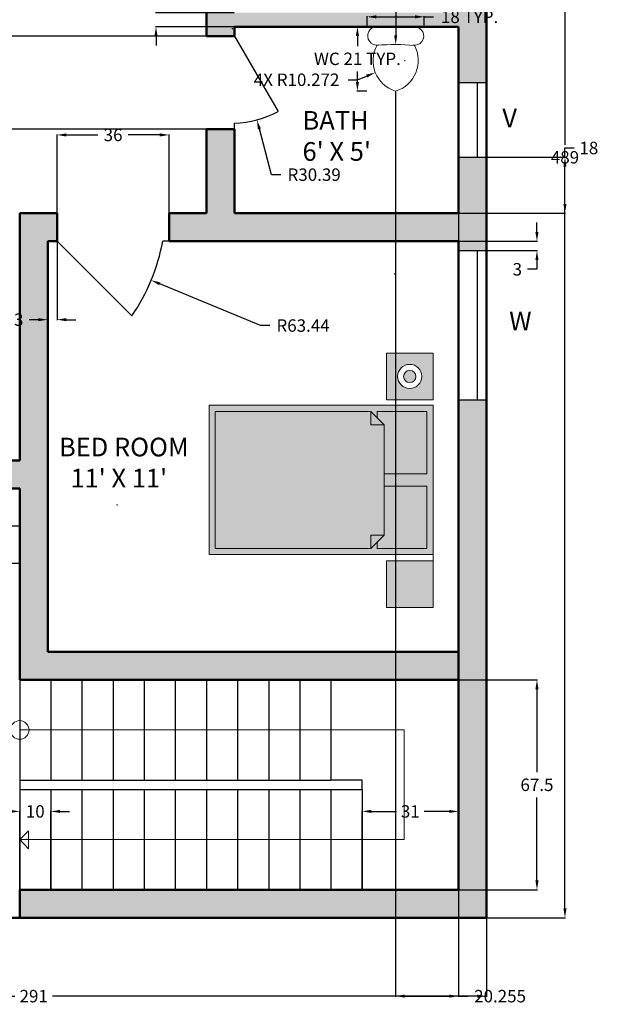
# Model space of a CAD drawing. Units: inches. Extents: x 30 to 385, y 81 to 626.
# Tile 2 of 4: x 199 to 385, y 81 to 398. Entities that reach past the tile are written whole.
import ezdxf

# ---------------------------------------------------------------- set-up
doc = ezdxf.new("R2010")
doc.units = ezdxf.units.IN
doc.header["$MEASUREMENT"] = 0
for name, color, linetype, lineweight in [('A-ANNO-DIMS', 2, 'Continuous', 18), ('A-ANNO-SYMB', 7, 'Continuous', 18), ('A-ANNO-TEXT', 7, 'Continuous', 18), ('A-AREA-IDEN', 7, 'Continuous', 25), ('A-DOOR', 3, 'Continuous', 25), ('A-FLOR-FIXT', 8, 'Continuous', 18), ('A-FLOR-STRS', 7, 'Continuous', 25), ('A-FURN', 8, 'Continuous', 18), ('A-GLAZ', 4, 'Continuous', 25), ('A-WALL', 7, 'Continuous', 50), ('A-WALL-PATT', 32, 'Continuous', 13)]:
    doc.layers.add(name, color=color, linetype=linetype, lineweight=lineweight)
doc.layers.add('A-FURN-PATT', color=254, linetype='Continuous', lineweight=13, true_color=0xfeeab9)
doc.styles.get("Standard").update_dxf_attribs({"font": 'arial.ttf'})
doc.dimstyles.get("Standard").update_dxf_attribs({"dimtxt": 4, "dimasz": 3, "dimexe": 0.18, "dimexo": 0.0625, "dimgap": 2, "dimtad": 0, "dimtih": 1, "dimtoh": 1, "dimdec": 0, "dimzin": 0, "dimdsep": 46, "dimlunit": 3, "dimtxsty": 'Standard', "dimcen": 0.09, "dimadec": 0, "dimazin": 0, "dimtfac": 1, "dimtdec": 0, "dimtofl": 0, "dimtmove": 0, "dimatfit": 3, "dimfxl": 1, "dimtolj": 1, "dimtzin": 0, "dimarcsym": 0})

# ---------------------------------------------------------------- blocks, each defined once
blk = doc.blocks.new('WIN-48')
for p, q in [((0, 0), (0, 9)), ((48, 0), (48, 9)), ((0, 6), (48, 6))]:
    blk.add_line(p, q)
blk = doc.blocks.new('VENT-24')
for p, q in [((0, 0), (9, 0)), ((6, 0), (6, -24)), ((0, -24), (9, -24))]:
    blk.add_line(p, q)
blk = doc.blocks.new('WC-TANK')
blk.add_line((0, 0), (-12, 0.05))
for centre, radius, start, end in [((-12.01, -2.95), 3, 89.7749, 278.744), ((-0.01, -3), 3, 260.8057, 89.7749), ((-3.03, -10.92), 10.27, 151.067, 252.7388), ((-6.31, -79.48), 73.74, 85.108, 94.4417), ((-9.05, -10.9), 10.27, 286.8109, 28.4828)]:
    blk.add_arc(centre, radius, start, end)
blk = doc.blocks.new('BED-48X72-WITH-NIGHTSTANDS')
for p, q in [((48, 0), (50, 0)), ((2, -2), (22, -2)), ((2, -18), (2, -2)), ((22, -2), (22, -15.76)), ((26, -2), (46, -2)), ((26, -2), (26, -15.76)), ((46, -2), (46, -18)), ((2, -20), (6.24, -15.76)), ((41.76, -15.76), (6.24, -15.76)), ((6.24, -15.76), (6.24, -20)), ((46, -20), (41.76, -15.76)), ((41.76, -15.76), (41.76, -20)), ((2, -18), (4, -18)), ((44, -18), (46, -18)), ((2, -20), (6.24, -20)), ((2, -70), (2, -20)), ((41.76, -20), (46, -20)), ((46, -20), (46, -70)), ((46, -70), (2, -70))]:
    blk.add_line(p, q)
for points in [[(-16.78, 0), (-1.78, 0), (-1.78, -15), (-16.78, -15)], [(0, 0), (48, 0), (48, -72), (0, -72)], [(50, 0), (65, 0), (65, -15), (50, -15)]]:
    blk.add_lwpolyline(points, close=True)
for radius in [3.89, 3.89, 3.89, 2]:
    blk.add_circle((-9.28, -7.5), radius)
blk = doc.blocks.new('*D10')
at = {"layer": 'A-ANNO-DIMS', "color": 0, "lineweight": -2, "transparency": 16777216}
for p, q in [((310.49, 395.62), (307.25, 395.62)), ((307.43, 392.62), (307.43, 389.29)), ((307.43, 377.83), (307.43, 381.16)), ((310.49, 374.83), (307.25, 374.83))]:
    blk.add_line(p, q, dxfattribs=at)
at = {"layer": 'A-ANNO-DIMS', "color": 0, "transparency": 16777216}
for points in [[(306.93, 392.62), (307.93, 392.62), (307.43, 395.62)], [(306.93, 377.83), (307.93, 377.83), (307.43, 374.83)]]:
    blk.add_solid(points, dxfattribs=at)
at = {"layer": 'Defpoints', "color": 0, "transparency": 16777216}
for p in [(307.43, 395.62), (310.55, 395.62), (310.55, 374.83)]:
    blk.add_point(p, dxfattribs=at)
at = {"layer": 'A-ANNO-DIMS', "color": 0, "transparency": 16777216, "insert": (307.43, 385.22), "char_height": 4, "attachment_point": 5}
blk.add_mtext('\\A1;WC 21 TYP.', dxfattribs=at)
blk = doc.blocks.new('*D11')
at = {"layer": 'A-ANNO-DIMS', "color": 0, "lineweight": -2, "transparency": 16777216}
for p, q in [((310.55, 395.68), (310.55, 398.91)), ((328.92, 395.68), (328.92, 398.91)), ((313.55, 398.73), (325.92, 398.73)), ((328.92, 398.73), (331.92, 398.73))]:
    blk.add_line(p, q, dxfattribs=at)
at = {"layer": 'A-ANNO-DIMS', "color": 0, "transparency": 16777216}
for points in [[(313.55, 399.23), (313.55, 398.23), (310.55, 398.73)], [(325.92, 399.23), (325.92, 398.23), (328.92, 398.73)]]:
    blk.add_solid(points, dxfattribs=at)
at = {"layer": 'Defpoints', "color": 0, "transparency": 16777216}
for p in [(328.92, 398.73), (310.55, 395.62), (328.92, 395.62)]:
    blk.add_point(p, dxfattribs=at)
at = {"layer": 'A-ANNO-DIMS', "color": 0, "transparency": 16777216, "insert": (343.47, 398.73), "char_height": 4, "attachment_point": 5}
blk.add_mtext('\\A1;18 TYP.', dxfattribs=at)
blk = doc.blocks.new('*D16')
at = {"layer": 'A-ANNO-DIMS', "color": 0, "lineweight": -2, "transparency": 16777216}
for p, q in [((57.92, 109), (57.92, 83.68)), ((348.92, 109), (348.92, 83.68)), ((60.92, 83.86), (197.35, 83.86)), ((345.92, 83.86), (209.49, 83.86))]:
    blk.add_line(p, q, dxfattribs=at)
at = {"layer": 'A-ANNO-DIMS', "color": 0, "transparency": 16777216}
for points in [[(60.92, 84.36), (60.92, 83.36), (57.92, 83.86)], [(345.92, 84.36), (345.92, 83.36), (348.92, 83.86)]]:
    blk.add_solid(points, dxfattribs=at)
at = {"layer": 'Defpoints', "color": 0, "transparency": 16777216}
for p in [(57.92, 109.06), (348.92, 109.06), (348.92, 83.86)]:
    blk.add_point(p, dxfattribs=at)
at = {"layer": 'A-ANNO-DIMS', "color": 0, "transparency": 16777216, "insert": (203.42, 83.86), "char_height": 4, "attachment_point": 5}
blk.add_mtext('\\A1;291', dxfattribs=at)
blk = doc.blocks.new('*D17')
at = {"layer": 'A-ANNO-DIMS', "color": 0, "lineweight": -2, "transparency": 16777216}
for p, q in [((348.98, 598.06), (374.3, 598.06)), ((374.12, 595.06), (374.12, 357.61)), ((374.12, 112.06), (374.12, 349.52)), ((348.98, 109.06), (374.3, 109.06))]:
    blk.add_line(p, q, dxfattribs=at)
at = {"layer": 'A-ANNO-DIMS', "color": 0, "transparency": 16777216}
for points in [[(373.62, 595.06), (374.62, 595.06), (374.12, 598.06)], [(373.62, 112.06), (374.62, 112.06), (374.12, 109.06)]]:
    blk.add_solid(points, dxfattribs=at)
at = {"layer": 'Defpoints', "color": 0, "transparency": 16777216}
for p in [(348.92, 598.06), (374.12, 598.06), (348.92, 109.06)]:
    blk.add_point(p, dxfattribs=at)
at = {"layer": 'A-ANNO-DIMS', "color": 0, "transparency": 16777216, "insert": (374.12, 353.56), "char_height": 4, "attachment_point": 5}
blk.add_mtext('\\A1;489', dxfattribs=at)
blk = doc.blocks.new('*D19')
at = {"layer": 'A-ANNO-DIMS', "color": 0, "lineweight": -2, "transparency": 16777216}
for p, q in [((339.98, 185.56), (365.3, 185.56)), ((365.12, 182.56), (365.12, 155.86)), ((365.12, 121.06), (365.12, 147.77)), ((339.98, 118.06), (365.3, 118.06))]:
    blk.add_line(p, q, dxfattribs=at)
at = {"layer": 'A-ANNO-DIMS', "color": 0, "transparency": 16777216}
for points in [[(364.62, 182.56), (365.62, 182.56), (365.12, 185.56)], [(364.62, 121.06), (365.62, 121.06), (365.12, 118.06)]]:
    blk.add_solid(points, dxfattribs=at)
at = {"layer": 'Defpoints', "color": 0, "transparency": 16777216}
for p in [(339.92, 185.56), (339.92, 118.06), (365.12, 118.06)]:
    blk.add_point(p, dxfattribs=at)
at = {"layer": 'A-ANNO-DIMS', "color": 0, "transparency": 16777216, "insert": (365.12, 151.81), "char_height": 4, "attachment_point": 5}
blk.add_mtext('\\A1;67.5', dxfattribs=at)
blk = doc.blocks.new('*D20')
at = {"layer": 'A-ANNO-DIMS', "color": 0, "lineweight": -2, "transparency": 16777216}
for p, q in [((365.12, 329.56), (365.12, 332.56)), ((339.98, 326.56), (365.3, 326.56)), ((339.98, 323.56), (365.3, 323.56)), ((365.12, 320.56), (365.12, 317.56)), ((365.12, 317.56), (362.12, 317.56))]:
    blk.add_line(p, q, dxfattribs=at)
at = {"layer": 'A-ANNO-DIMS', "color": 0, "transparency": 16777216}
for points in [[(364.62, 329.56), (365.62, 329.56), (365.12, 326.56)], [(364.62, 320.56), (365.62, 320.56), (365.12, 323.56)]]:
    blk.add_solid(points, dxfattribs=at)
at = {"layer": 'Defpoints', "color": 0, "transparency": 16777216}
for p in [(339.92, 326.56), (339.92, 323.56), (365.12, 323.56)]:
    blk.add_point(p, dxfattribs=at)
at = {"layer": 'A-ANNO-DIMS', "color": 0, "transparency": 16777216, "insert": (358.81, 317.56), "char_height": 4, "attachment_point": 5}
blk.add_mtext('\\A1;3', dxfattribs=at)
blk = doc.blocks.new('*D21')
at = {"layer": 'A-ANNO-DIMS', "color": 0, "lineweight": -2, "transparency": 16777216}
for p, q in [((374.12, 353.56), (374.12, 356.56)), ((374.12, 356.56), (377.12, 356.56)), ((339.98, 353.56), (374.3, 353.56)), ((374.12, 338.56), (374.12, 350.56)), ((339.98, 335.56), (374.3, 335.56))]:
    blk.add_line(p, q, dxfattribs=at)
at = {"layer": 'A-ANNO-DIMS', "color": 0, "transparency": 16777216}
for points in [[(373.62, 350.56), (374.62, 350.56), (374.12, 353.56)], [(373.62, 338.56), (374.62, 338.56), (374.12, 335.56)]]:
    blk.add_solid(points, dxfattribs=at)
at = {"layer": 'Defpoints', "color": 0, "transparency": 16777216}
for p in [(339.92, 353.56), (374.12, 353.56), (339.92, 335.56)]:
    blk.add_point(p, dxfattribs=at)
at = {"layer": 'A-ANNO-DIMS', "color": 0, "transparency": 16777216, "insert": (381.8, 356.56), "char_height": 4, "attachment_point": 5}
blk.add_mtext('\\A1;18', dxfattribs=at)
blk = doc.blocks.new('*D36')
at = {"layer": 'A-ANNO-DIMS', "color": 0, "lineweight": -2, "transparency": 16777216}
for p, q in [((210.92, 335.63), (210.92, 360.94)), ((246.92, 335.63), (246.92, 360.94)), ((213.92, 360.76), (224.06, 360.76)), ((243.92, 360.76), (233.78, 360.76))]:
    blk.add_line(p, q, dxfattribs=at)
at = {"layer": 'A-ANNO-DIMS', "color": 0, "transparency": 16777216}
for points in [[(213.92, 361.26), (213.92, 360.26), (210.92, 360.76)], [(243.92, 361.26), (243.92, 360.26), (246.92, 360.76)]]:
    blk.add_solid(points, dxfattribs=at)
at = {"layer": 'Defpoints', "color": 0, "transparency": 16777216}
for p in [(246.92, 360.76), (210.92, 335.56), (246.92, 335.56)]:
    blk.add_point(p, dxfattribs=at)
at = {"layer": 'A-ANNO-DIMS', "color": 0, "transparency": 16777216, "insert": (228.92, 360.76), "char_height": 4, "attachment_point": 5}
blk.add_mtext('\\A1;36', dxfattribs=at)
blk = doc.blocks.new('*D37')
at = {"layer": 'A-ANNO-DIMS', "color": 0, "lineweight": -2, "transparency": 16777216}
for p, q in [((207.92, 326.5), (207.92, 301.18)), ((210.92, 326.5), (210.92, 301.18)), ((204.92, 301.36), (201.92, 301.36)), ((213.92, 301.36), (216.92, 301.36))]:
    blk.add_line(p, q, dxfattribs=at)
at = {"layer": 'A-ANNO-DIMS', "color": 0, "transparency": 16777216}
for points in [[(204.92, 301.86), (204.92, 300.86), (207.92, 301.36)], [(213.92, 301.86), (213.92, 300.86), (210.92, 301.36)]]:
    blk.add_solid(points, dxfattribs=at)
at = {"layer": 'Defpoints', "color": 0, "transparency": 16777216}
for p in [(207.92, 326.56), (210.92, 326.56), (207.92, 301.36)]:
    blk.add_point(p, dxfattribs=at)
at = {"layer": 'A-ANNO-DIMS', "color": 0, "transparency": 16777216, "insert": (198.61, 301.36), "char_height": 4, "attachment_point": 5}
blk.add_mtext('\\A1;3', dxfattribs=at)
blk = doc.blocks.new('*D40')
at = {"layer": 'A-ANNO-DIMS', "color": 0, "lineweight": -2, "transparency": 16777216}
for p, q in [((258.86, 392.56), (32.54, 392.56)), ((32.72, 389.56), (32.72, 381.61)), ((32.72, 365.56), (32.72, 373.52)), ((258.86, 362.56), (32.54, 362.56))]:
    blk.add_line(p, q, dxfattribs=at)
at = {"layer": 'A-ANNO-DIMS', "color": 0, "transparency": 16777216}
for points in [[(32.22, 389.56), (33.22, 389.56), (32.72, 392.56)], [(32.22, 365.56), (33.22, 365.56), (32.72, 362.56)]]:
    blk.add_solid(points, dxfattribs=at)
at = {"layer": 'Defpoints', "color": 0, "transparency": 16777216}
for p in [(32.72, 392.56), (258.92, 392.56), (258.92, 362.56)]:
    blk.add_point(p, dxfattribs=at)
at = {"layer": 'A-ANNO-DIMS', "color": 0, "transparency": 16777216, "insert": (32.72, 377.56), "char_height": 4, "attachment_point": 5}
blk.add_mtext('\\A1;30', dxfattribs=at)
blk = doc.blocks.new('*D41')
at = {"layer": 'A-ANNO-DIMS', "color": 0, "lineweight": -2, "transparency": 16777216}
for p, q in [((242.72, 403.06), (242.72, 406.06)), ((242.72, 406.06), (245.72, 406.06)), ((267.86, 400.06), (242.54, 400.06)), ((267.86, 395.56), (242.54, 395.56)), ((242.72, 392.56), (242.72, 389.56))]:
    blk.add_line(p, q, dxfattribs=at)
at = {"layer": 'A-ANNO-DIMS', "color": 0, "transparency": 16777216}
for points in [[(242.22, 403.06), (243.22, 403.06), (242.72, 400.06)], [(242.22, 392.56), (243.22, 392.56), (242.72, 395.56)]]:
    blk.add_solid(points, dxfattribs=at)
at = {"layer": 'Defpoints', "color": 0, "transparency": 16777216}
for p in [(242.72, 400.06), (267.92, 400.06), (267.92, 395.56)]:
    blk.add_point(p, dxfattribs=at)
at = {"layer": 'A-ANNO-DIMS', "color": 0, "transparency": 16777216, "insert": (251.46, 406.06), "char_height": 4, "attachment_point": 5}
blk.add_mtext('\\A1;4.5', dxfattribs=at)
blk = doc.blocks.new('*D43')
at = {"layer": 'A-ANNO-DIMS', "color": 0, "lineweight": -2, "transparency": 16777216}
for p, q in [((339.92, 377.5), (339.92, 83.68)), ((319.66, 374.77), (319.66, 83.68)), ((322.66, 83.86), (336.92, 83.86)), ((339.92, 83.86), (342.92, 83.86))]:
    blk.add_line(p, q, dxfattribs=at)
at = {"layer": 'A-ANNO-DIMS', "color": 0, "transparency": 16777216}
for points in [[(322.66, 84.36), (322.66, 83.36), (319.66, 83.86)], [(336.92, 84.36), (336.92, 83.36), (339.92, 83.86)]]:
    blk.add_solid(points, dxfattribs=at)
at = {"layer": 'Defpoints', "color": 0, "transparency": 16777216}
for p in [(339.92, 377.56), (319.66, 374.83), (339.92, 83.86)]:
    blk.add_point(p, dxfattribs=at)
at = {"layer": 'A-ANNO-DIMS', "color": 0, "transparency": 16777216, "insert": (353.27, 83.86), "char_height": 4, "attachment_point": 5}
blk.add_mtext('\\A1;20.255', dxfattribs=at)
blk = doc.blocks.new('*D44')
at = {"layer": 'A-ANNO-DIMS', "color": 0, "lineweight": -2, "transparency": 16777216}
for p, q in [((308.92, 118.13), (308.92, 143.44)), ((311.92, 143.26), (319.94, 143.26)), ((336.92, 143.26), (328.9, 143.26)), ((339.92, 118.13), (339.92, 143.44))]:
    blk.add_line(p, q, dxfattribs=at)
at = {"layer": 'A-ANNO-DIMS', "color": 0, "transparency": 16777216}
for points in [[(311.92, 143.76), (311.92, 142.76), (308.92, 143.26)], [(336.92, 143.76), (336.92, 142.76), (339.92, 143.26)]]:
    blk.add_solid(points, dxfattribs=at)
at = {"layer": 'Defpoints', "color": 0, "transparency": 16777216}
for p in [(339.92, 143.26), (308.92, 118.06), (339.92, 118.06)]:
    blk.add_point(p, dxfattribs=at)
at = {"layer": 'A-ANNO-DIMS', "color": 0, "transparency": 16777216, "insert": (324.42, 143.26), "char_height": 4, "attachment_point": 5}
blk.add_mtext('\\A1;31', dxfattribs=at)
blk = doc.blocks.new('*D46')
at = {"layer": 'A-ANNO-DIMS', "color": 0, "lineweight": -2, "transparency": 16777216}
for p, q in [((195.919029, 143.263849), (192.919029, 143.263849)), ((198.919029, 118.126349), (198.919029, 143.443849)), ((208.919029, 118.126349), (208.919029, 143.443849)), ((211.919029, 143.263849), (214.919029, 143.263849))]:
    blk.add_line(p, q, dxfattribs=at)
at = {"layer": 'A-ANNO-DIMS', "color": 0, "transparency": 16777216}
for points in [[(195.919029, 143.763849), (195.919029, 142.763849), (198.919029, 143.263849)], [(211.919029, 143.763849), (211.919029, 142.763849), (208.919029, 143.263849)]]:
    blk.add_solid(points, dxfattribs=at)
at = {"layer": 'Defpoints', "color": 0, "transparency": 16777216}
for p in [(208.919029, 143.263849), (198.919029, 118.063849), (208.919029, 118.063849)]:
    blk.add_point(p, dxfattribs=at)
at = {"layer": 'A-ANNO-DIMS', "color": 0, "transparency": 16777216, "insert": (203.919029, 143.263849), "char_height": 4, "attachment_point": 5}
blk.add_mtext('\\A1;10', dxfattribs=at)
blk = doc.blocks.new('*D54')
at = {"layer": 'A-ANNO-DIMS', "color": 0, "lineweight": -2, "transparency": 16777216}
for p, q in [((106.69, 291.78), (109.69, 291.78)), ((109.69, 291.78), (152.14, 274.2)), ((230.19, 241.83), (230.37, 241.83)), ((230.28, 241.74), (230.28, 241.92))]:
    blk.add_line(p, q, dxfattribs=at)
at = {"layer": 'A-ANNO-DIMS', "color": 0, "transparency": 16777216}
blk.add_solid([(152.33, 274.66), (151.95, 273.74), (154.91, 273.05)], dxfattribs=at)
at = {"layer": 'Defpoints', "color": 0, "transparency": 16777216}
for p in [(154.91, 273.05), (230.28, 241.83)]:
    blk.add_point(p, dxfattribs=at)
at = {"layer": 'A-ANNO-DIMS', "color": 0, "transparency": 16777216, "insert": (96.02, 291.78), "char_height": 4, "attachment_point": 5}
blk.add_mtext('\\A1;R81.58', dxfattribs=at)
blk = doc.blocks.new('*D55')
at = {"layer": 'A-ANNO-DIMS', "color": 0, "lineweight": -2, "transparency": 16777216}
for p, q in [((182.46, 338.32), (182.64, 338.32)), ((182.55, 338.23), (182.55, 338.41)), ((276.32, 299.47), (243.93, 312.89)), ((279.32, 299.47), (276.32, 299.47))]:
    blk.add_line(p, q, dxfattribs=at)
at = {"layer": 'A-ANNO-DIMS', "color": 0, "transparency": 16777216}
blk.add_solid([(244.12, 313.35), (243.73, 312.43), (241.15, 314.04)], dxfattribs=at)
at = {"layer": 'Defpoints', "color": 0, "transparency": 16777216}
for p in [(182.55, 338.32), (241.15, 314.04)]:
    blk.add_point(p, dxfattribs=at)
at = {"layer": 'A-ANNO-DIMS', "color": 0, "transparency": 16777216, "insert": (289.97, 299.47), "char_height": 4, "attachment_point": 5}
blk.add_mtext('\\A1;R63.44', dxfattribs=at)
blk = doc.blocks.new('*D57')
at = {"layer": 'A-ANNO-DIMS', "color": 0, "lineweight": -2, "transparency": 16777216}
for p, q in [((267.19, 394.95), (267.37, 394.95)), ((267.28, 394.86), (267.28, 395.04)), ((279.87, 347.98), (275.92, 362.7)), ((282.87, 347.98), (279.87, 347.98))]:
    blk.add_line(p, q, dxfattribs=at)
at = {"layer": 'A-ANNO-DIMS', "color": 0, "transparency": 16777216}
blk.add_solid([(276.41, 362.82), (275.44, 362.57), (275.15, 365.59)], dxfattribs=at)
at = {"layer": 'Defpoints', "color": 0, "transparency": 16777216}
for p in [(267.28, 394.95), (275.15, 365.59)]:
    blk.add_point(p, dxfattribs=at)
at = {"layer": 'A-ANNO-DIMS', "color": 0, "transparency": 16777216, "insert": (293.53, 347.98), "char_height": 4, "attachment_point": 5}
blk.add_mtext('\\A1;R30.39', dxfattribs=at)
blk = doc.blocks.new('*D59')
at = {"layer": 'A-ANNO-DIMS', "color": 0, "lineweight": -2, "transparency": 16777216}
for p, q in [((319.9, 434.08), (319.73, 392.83)), ((322.9, 434.08), (319.9, 434.08)), ((319.34, 316.09), (319.52, 316.09)), ((319.43, 316), (319.43, 316.18))]:
    blk.add_line(p, q, dxfattribs=at)
at = {"layer": 'A-ANNO-DIMS', "color": 0, "transparency": 16777216}
blk.add_solid([(319.23, 392.83), (320.23, 392.83), (319.72, 389.83)], dxfattribs=at)
at = {"layer": 'Defpoints', "color": 0, "transparency": 16777216}
for p in [(319.72, 389.83), (319.43, 316.09)]:
    blk.add_point(p, dxfattribs=at)
at = {"layer": 'A-ANNO-DIMS', "color": 0, "transparency": 16777216, "insert": (337.88, 434.08), "char_height": 4, "attachment_point": 5}
blk.add_mtext('\\A1;2X R73.74', dxfattribs=at)
blk = doc.blocks.new('*D60')
at = {"layer": 'A-ANNO-DIMS', "color": 0, "lineweight": -2, "transparency": 16777216}
for p, q in [((322.62, 384.64), (322.8, 384.64)), ((322.71, 384.55), (322.71, 384.73)), ((304.46, 378.51), (307.46, 378.51)), ((307.46, 378.51), (310.4, 379.69))]:
    blk.add_line(p, q, dxfattribs=at)
at = {"layer": 'A-ANNO-DIMS', "color": 0, "transparency": 16777216}
blk.add_solid([(310.21, 380.15), (310.58, 379.23), (313.18, 380.81)], dxfattribs=at)
at = {"layer": 'Defpoints', "color": 0, "transparency": 16777216}
for p in [(322.71, 384.64), (313.18, 380.81)]:
    blk.add_point(p, dxfattribs=at)
at = {"layer": 'A-ANNO-DIMS', "color": 0, "transparency": 16777216, "insert": (287.89, 378.51), "char_height": 4, "attachment_point": 5}
blk.add_mtext('\\A1;4X R10.272', dxfattribs=at)

msp = doc.modelspace()

# ---------------------------------------------------------------- hatches: boundary and pattern name
at = {"layer": 'A-FURN-PATT'}
h = msp.add_hatch(color=256, dxfattribs=at)
h.paths.add_polyline_path([(259.7424, 273.8309), (259.7424, 225.8309), (331.7424, 225.8309), (331.7424, 273.8309)])
h.paths.add_polyline_path([(313.7424, 271.8309), (329.7424, 271.8309), (329.7424, 251.8309), (315.9851, 251.8309), (315.9851, 247.8309), (329.7424, 247.8309), (329.7424, 227.8309), (313.7424, 227.8309), (313.7424, 229.8309), (311.7424, 227.8309), (261.7424, 227.8309), (261.7424, 271.8309), (311.7424, 271.8309), (313.7424, 269.8309)], flags=16)
h.paths.add_polyline_path([(316.7424, 208.8309), (331.7424, 208.8309), (331.7424, 223.8309), (316.7424, 223.8309)])
h.paths.add_polyline_path([(316.7424, 275.6141), (331.7424, 275.6141), (331.7424, 290.6141), (316.7424, 290.6141)])
h.paths.add_polyline_path([(320.351, 283.1141, -1), (328.1339, 283.1141, -1)], flags=16)
h.paths.add_polyline_path([(322.2424, 283.1141, -1), (326.2424, 283.1141, -1)], flags=0)
h = msp.add_hatch(color=256, dxfattribs=at)
h.paths.add_polyline_path([(311.7424, 227.8309), (311.7424, 232.0735), (315.9851, 232.0735), (315.9851, 267.5882), (311.7424, 267.5882), (311.7424, 271.8309), (261.7424, 271.8309), (261.7424, 227.8309)])
h.paths.add_polyline_path([(315.9851, 232.0735), (311.7424, 232.0735), (311.7424, 227.8309)], flags=17)
h.paths.add_polyline_path([(315.9851, 267.5882), (311.7424, 271.8309), (311.7424, 267.5882)], flags=17)
h = msp.add_hatch(color=256, dxfattribs=at)
h.paths.add_polyline_path([(315.9851, 251.8309), (329.7424, 251.8309), (329.7424, 271.8309), (313.7424, 271.8309), (313.7424, 269.8309), (315.9851, 267.5882)])
h.paths.add_polyline_path([(315.9851, 247.8309), (315.9851, 232.0735), (313.7424, 229.8309), (313.7424, 227.8309), (329.7424, 227.8309), (329.7424, 247.8309)])
at = {"layer": 'A-WALL-PATT'}
h = msp.add_hatch(color=256, dxfattribs=at)
h.paths.add_polyline_path([(66.919, 385.0638), (57.919, 385.0638), (57.919, 331.0638), (60.919, 331.0638), (66.919, 331.0638)])
h.paths.add_polyline_path([(306.919, 469.0638), (249.919, 469.0638), (249.919, 460.0638), (258.919, 460.0638), (258.919, 392.5638), (267.919, 392.5638), (267.919, 395.5638), (339.919, 395.5638), (339.919, 377.5638), (348.919, 377.5638), (348.919, 418.0638), (339.919, 418.0638), (339.919, 400.0638), (267.919, 400.0638), (267.919, 460.0638), (306.919, 460.0638)])
h.paths.add_polyline_path([(339.919, 194.5638), (207.919, 194.5638), (207.919, 326.5638), (210.919, 326.5638), (210.919, 335.5638), (198.919, 335.5638), (198.919, 256.0638), (195.919, 256.0638), (195.919, 247.0638), (198.919, 247.0638), (198.919, 194.5638), (198.919, 185.5638), (339.919, 185.5638)])
msp.add_hatch(color=256, dxfattribs=at).paths.add_polyline_path([(348.919, 353.5638), (339.919, 353.5638), (339.919, 335.5638), (267.919, 335.5638), (267.919, 362.5638), (258.919, 362.5638), (258.919, 335.5638), (246.919, 335.5638), (246.919, 326.5638), (339.919, 326.5638), (339.919, 323.5638), (348.919, 323.5638)])
h = msp.add_hatch(color=256, dxfattribs=at)
h.paths.add_polyline_path([(66.919, 283.0638), (57.919, 283.0638), (57.919, 247.0638), (66.919, 247.0638), (135.919, 247.0638), (135.919, 256.0638), (66.919, 256.0638)])
h.paths.add_polyline_path([(348.919, 275.5638), (339.919, 275.5638), (339.919, 118.0638), (198.919, 118.0638), (198.919, 109.0638), (348.919, 109.0638)])

# ---------------------------------------------------------------- linework, layer by layer
at = {"layer": 'A-ANNO-SYMB'}
for p, q in [((208.919, 169.4388), (198.919, 169.4388)), ((208.919, 169.4388), (322.502, 169.4388)), ((322.502, 169.4388), (322.502, 134.1888)), ((198.919, 134.1888), (201.7475, 137.0173)), ((201.7475, 137.0173), (201.7475, 134.1888)), ((322.502, 134.1888), (198.919, 134.1888)), ((201.7475, 131.1888), (198.919, 134.1888)), ((201.7475, 134.1888), (201.7475, 131.1888))]:
    msp.add_line(p, q, dxfattribs=at)
msp.add_circle((198.919, 169.4388), 3, dxfattribs=at)
at = {"layer": 'A-DOOR'}
for p, q in [((267.919, 392.5638), (281.9188, 368.3155)), ((267.919, 362.5638), (267.919, 364.5643)), ((210.919, 326.5638), (234.9365, 302.5464)), ((246.919, 326.5638), (244.8849, 326.5638))]:
    msp.add_line(p, q, dxfattribs=at)
for centre, radius, start, end in [((267.2805, 394.9469), 30.3893, 271.203977, 298.796023), ((182.5453, 338.3166), 63.4378, 325.67657, 349.32343)]:
    msp.add_arc(centre, radius, start, end, dxfattribs=at)
at = {"layer": 'A-FLOR-STRS'}
for p, q in [((126.919, 235.0638), (198.919, 235.0638)), ((126.919, 223.0638), (198.919, 223.0638)), ((198.919, 185.5638), (198.919, 118.0638)), ((208.919, 185.5638), (208.919, 153.3138)), ((218.919, 185.5638), (218.919, 153.3138)), ((228.919, 185.5638), (228.919, 153.3138)), ((238.919, 185.5638), (238.919, 153.3138)), ((248.919, 185.5638), (248.919, 153.3138)), ((258.919, 185.5638), (258.919, 153.3138)), ((268.919, 185.5638), (268.919, 153.3138)), ((278.919, 185.5638), (278.919, 153.3138)), ((288.919, 185.5638), (288.919, 153.3138)), ((298.919, 185.5638), (298.919, 153.3138)), ((198.919, 153.3138), (298.919, 153.3138)), ((308.919, 153.3138), (298.919, 153.3138)), ((308.919, 150.3138), (308.919, 153.3138)), ((198.919, 150.3138), (298.919, 150.3138)), ((208.919, 150.3138), (208.919, 118.0638)), ((218.919, 150.3138), (218.919, 118.0638)), ((228.919, 150.3138), (228.919, 118.0638)), ((238.919, 150.3138), (238.919, 118.0638)), ((248.919, 150.3138), (248.919, 118.0638)), ((258.919, 150.3138), (258.919, 118.0638)), ((268.919, 150.3138), (268.919, 118.0638)), ((278.919, 150.3138), (278.919, 118.0638)), ((288.919, 150.3138), (288.919, 118.0638)), ((298.919, 150.3138), (308.919, 150.3138)), ((298.919, 150.3138), (298.919, 118.0638)), ((308.919, 150.3138), (308.919, 118.0638))]:
    msp.add_line(p, q, dxfattribs=at)
at = {"layer": 'A-WALL'}
for p, q in [((348.919, 109.0638), (348.919, 598.0638)), ((258.919, 392.5638), (258.919, 460.0638)), ((267.919, 392.5638), (258.919, 392.5638)), ((339.919, 395.5638), (267.919, 395.5638)), ((267.919, 392.5638), (267.919, 395.5638)), ((339.919, 335.5638), (339.919, 395.5638)), ((258.919, 335.5638), (258.919, 362.5638)), ((267.919, 362.5638), (258.919, 362.5638)), ((267.919, 335.5638), (267.919, 362.5638)), ((198.919, 335.5638), (198.919, 256.0638)), ((210.919, 335.5638), (198.919, 335.5638)), ((210.919, 326.5638), (210.919, 335.5638)), ((258.919, 335.5638), (246.919, 335.5638)), ((246.919, 326.5638), (246.919, 335.5638)), ((339.919, 335.5638), (267.919, 335.5638)), ((207.919, 194.5638), (207.919, 326.5638)), ((210.919, 326.5638), (207.919, 326.5638)), ((339.919, 326.5638), (246.919, 326.5638)), ((339.919, 118.0638), (339.919, 326.5638)), ((198.919, 256.0638), (195.919, 256.0638)), ((198.919, 247.0638), (195.919, 247.0638)), ((198.919, 247.0638), (198.919, 194.5638)), ((198.919, 194.5638), (198.919, 185.5638)), ((339.919, 194.5638), (207.919, 194.5638)), ((339.919, 185.5638), (198.919, 185.5638)), ((198.919, 118.0638), (339.919, 118.0638)), ((198.919, 118.0638), (198.919, 109.0638)), ((57.919, 109.0638), (348.919, 109.0638))]:
    msp.add_line(p, q, dxfattribs=at)

# ---------------------------------------------------------------- block references
at = {"layer": 'A-FLOR-FIXT'}
msp.add_blockref('WC-TANK', (325.7451, 395.5638), dxfattribs=at)
at = {"layer": 'A-FURN', "rotation": 269.9999999999999}
msp.add_blockref('BED-48X72-WITH-NIGHTSTANDS', (331.7424, 273.8309), dxfattribs=at)
at = {"layer": 'A-GLAZ'}
msp.add_blockref('VENT-24', (339.919, 377.5638), dxfattribs=at)
at = {"layer": 'A-GLAZ', "rotation": 270.0000000000001}
msp.add_blockref('WIN-48', (339.919, 323.5638), dxfattribs=at)

# ---------------------------------------------------------------- texts
at = {"layer": 'A-ANNO-TEXT', "char_height": 6, "attachment_point": 1}
for s, insert in [('V', (353.9861, 369.2206)), ('W', (356.2033, 303.9283))]:
    msp.add_mtext_dynamic_manual_height_columns(s, width=76.086845, gutter_width=1, heights=[0], dxfattribs=dict(at, insert=insert))
at = {"layer": 'A-AREA-IDEN', "char_height": 6, "attachment_point": 1}
for s, insert in [("  BATH\\P  6' X 5'", (286.1242, 368.4452)), ("BED ROOM\\P  11' X 11'", (211.5543, 263.4101))]:
    msp.add_mtext_dynamic_manual_height_columns(s, width=76.086845, gutter_width=1, heights=[0], dxfattribs=dict(at, insert=insert))

# ---------------------------------------------------------------- dimensions: what is measured, and where the dimension line sits
at = {"layer": 'A-ANNO-DIMS'}
for base, p1, p2, angle, override, picture, middle in [((374.119, 598.0638), (348.919, 109.0638), (348.919, 598.0638), 90, {"dimdec": 0, "dimlfac": 1, "dimrnd": 0, "dimzin": 0, "dimdsep": 46, "dimlunit": 2}, '*D17', (374.119, 353.5638)), ((242.719, 400.0638), (267.919, 395.5638), (267.919, 400.0638), 90, {"dimdec": 1, "dimlfac": 1, "dimrnd": 0, "dimzin": 0, "dimdsep": 46, "dimlunit": 2}, '*D41', (251.4557, 406.0638)), ((32.719, 392.5638), (258.919, 362.5638), (258.919, 392.5638), 90, {"dimdec": 0, "dimlfac": 1, "dimrnd": 0, "dimzin": 0, "dimdsep": 46, "dimlunit": 2}, '*D40', (32.719, 377.5638)), ((374.119, 353.5638), (339.919, 335.5638), (339.919, 353.5638), 90, {"dimdec": 0, "dimlfac": 1, "dimrnd": 0, "dimzin": 0, "dimdsep": 46, "dimlunit": 2}, '*D21', (381.7998, 356.5638)), ((365.119, 323.5638), (339.919, 326.5638), (339.919, 323.5638), 270, {"dimdec": 0, "dimlfac": 1, "dimrnd": 0, "dimzin": 0, "dimdsep": 46, "dimlunit": 2}, '*D20', (358.8093, 317.5638)), ((207.919, 301.3638), (210.919, 326.5638), (207.919, 326.5638), 180, {"dimdec": 0, "dimlfac": 1, "dimrnd": 0, "dimzin": 0, "dimdsep": 46, "dimlunit": 2}, '*D37', (198.6093, 301.3638)), ((365.119, 118.0638), (339.919, 185.5638), (339.919, 118.0638), 270, {"dimdec": 1, "dimlfac": 1, "dimrnd": 0, "dimzin": 0, "dimdsep": 46, "dimlunit": 2}, '*D19', (365.119, 151.8138))]:
    dim = msp.add_linear_dim(base=base, p1=p1, p2=p2, angle=angle, dimstyle='Standard', override=override, dxfattribs=at)
    dim.commit()
    dim.dimension.update_dxf_attribs({"geometry": picture, "text_midpoint": middle})
for center, mpoint, text, override, picture, middle in [((319.4328, 316.0876), (319.723, 389.832), '2X <>', {"dimdec": 2, "dimlfac": 1, "dimrnd": 0, "dimzin": 0, "dimdsep": 46, "dimlunit": 2}, '*D59', (337.8835, 434.0786)), ((322.7116, 384.6415), (313.1809, 380.8099), '4X <>', {"dimdec": 3, "dimlfac": 1, "dimrnd": 0, "dimzin": 0, "dimdsep": 46, "dimlunit": 2}, '*D60', (287.8881, 378.511))]:
    dim = msp.add_radius_dim(center=center, mpoint=mpoint, text=text, dimstyle='Standard', override=override, dxfattribs=at)
    dim.commit()
    dim.dimension.update_dxf_attribs({"geometry": picture, "text_midpoint": middle, "dimtype": 164})
dim = msp.add_linear_dim(base=(328.9197, 398.7329), p1=(310.5498, 395.6154), p2=(328.9197, 395.6154), text='<> TYP.', dimstyle='Standard', override={"dimdec": 0, "dimlfac": 1, "dimrnd": 0, "dimzin": 0, "dimdsep": 46, "dimlunit": 2}, dxfattribs=at)
dim.commit()
dim.dimension.update_dxf_attribs({"geometry": '*D11', "text_midpoint": (343.4668, 398.7329)})
for center, mpoint, picture, middle in [((267.2805, 394.9469), (275.146, 365.5931), '*D57', (293.5324, 347.9808)), ((182.5453, 338.3166), (241.1541, 314.0399), '*D55', (289.9743, 299.4739)), ((230.2759, 241.8327), (154.9082, 273.0509), '*D54', (96.0204, 291.7818))]:
    dim = msp.add_radius_dim(center=center, mpoint=mpoint, dimstyle='Standard', override={"dimdec": 2, "dimlfac": 1, "dimrnd": 0, "dimzin": 0, "dimdsep": 46, "dimlunit": 2}, dxfattribs=at)
    dim.commit()
    dim.dimension.update_dxf_attribs({"geometry": picture, "text_midpoint": middle, "dimtype": 164})
dim = msp.add_linear_dim(base=(307.4323, 395.6154), p1=(310.5498, 374.8321), p2=(310.5498, 395.6154), angle=90, text='WC <> TYP.', dimstyle='Standard', override={"dimdec": 0, "dimlfac": 1, "dimrnd": 0, "dimzin": 0, "dimdsep": 46, "dimlunit": 2}, dxfattribs=at)
dim.commit()
dim.dimension.update_dxf_attribs({"geometry": '*D10', "text_midpoint": (307.4323, 385.2238)})
for base, p1, p2, override, picture, middle in [((339.919, 83.8638), (319.6636, 374.8321), (339.919, 377.5638), {"dimdec": 3, "dimlfac": 1, "dimrnd": 0, "dimzin": 0, "dimdsep": 46, "dimlunit": 2}, '*D43', (353.271, 83.8638)), ((246.919, 360.7638), (210.919, 335.5638), (246.919, 335.5638), {"dimdec": 0, "dimlfac": 1, "dimrnd": 0, "dimzin": 0, "dimdsep": 46, "dimlunit": 2}, '*D36', (228.919, 360.7638)), ((208.919, 143.2638), (198.919, 118.0638), (208.919, 118.0638), {"dimdec": 0, "dimlfac": 1, "dimrnd": 0, "dimzin": 0, "dimdsep": 46, "dimlunit": 2}, '*D46', (203.919, 143.2638)), ((339.919, 143.2638), (308.919, 118.0638), (339.919, 118.0638), {"dimdec": 0, "dimlfac": 1, "dimrnd": 0, "dimzin": 0, "dimdsep": 46, "dimlunit": 2}, '*D44', (324.419, 143.2638)), ((348.919, 83.8638), (57.919, 109.0638), (348.919, 109.0638), {"dimdec": 0, "dimlfac": 1, "dimrnd": 0, "dimzin": 0, "dimdsep": 46, "dimlunit": 2}, '*D16', (203.419, 83.8638))]:
    dim = msp.add_linear_dim(base=base, p1=p1, p2=p2, dimstyle='Standard', override=override, dxfattribs=at)
    dim.commit()
    dim.dimension.update_dxf_attribs({"geometry": picture, "text_midpoint": middle})

doc.saveas('drawing.dxf')
